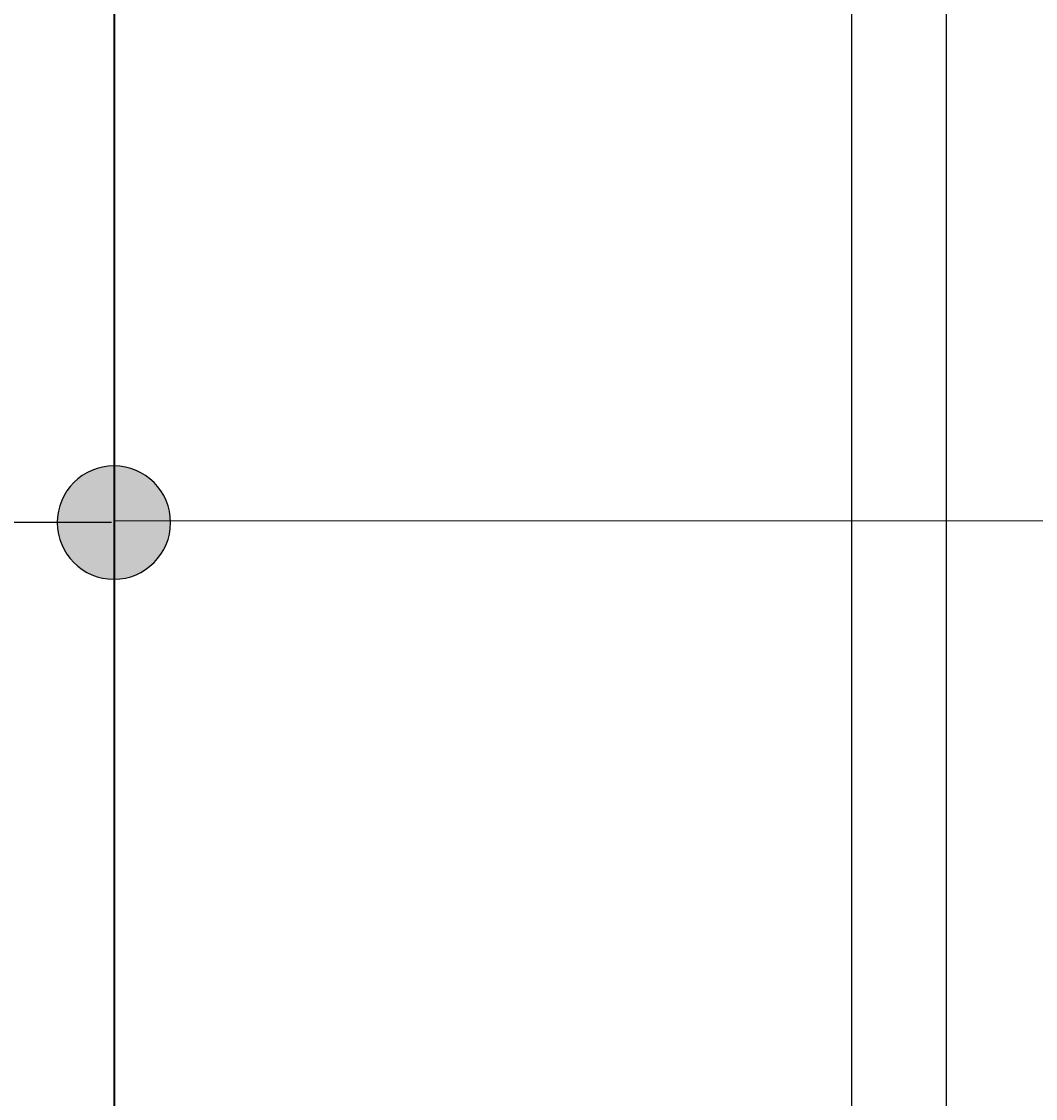
# Model space of a CAD drawing. Units: inches. Extents: x 738 to 1068, y 378 to 757.
# Tile 25 of 41: x 779 to 806, y 578 to 606. Entities that reach past the tile are written whole.
import ezdxf

# ---------------------------------------------------------------- set-up
doc = ezdxf.new("R2010")
doc.units = ezdxf.units.IN
doc.header["$MEASUREMENT"] = 0
for name, color, linetype, lineweight in [('A-ANNO-DIMS', 2, 'Continuous', 18), ('E-CONN', 7, 'Continuous', 25), ('E-CONN-PATT', 7, 'Continuous', 13), ('E-CTRL-WIRE', 7, 'Continuous', 18), ('E-POWR-FEED', 7, 'Continuous', 35)]:
    doc.layers.add(name, color=color, linetype=linetype, lineweight=lineweight)
doc.styles.get("Standard").update_dxf_attribs({"font": 'arial.ttf'})
doc.dimstyles.get("Standard").update_dxf_attribs({"dimtxt": 0.18, "dimasz": 0.18, "dimexe": 0.18, "dimexo": 0.0625, "dimgap": 0.09, "dimtad": 0, "dimtih": 1, "dimtoh": 1, "dimdec": 4, "dimzin": 0, "dimdsep": 46, "dimtxsty": 'Standard', "dimcen": 0.09, "dimadec": 0, "dimazin": 0, "dimtfac": 1, "dimtdec": 4, "dimtofl": 0, "dimtmove": 0, "dimatfit": 3, "dimfxl": 1, "dimtolj": 1, "dimtzin": 0, "dimarcsym": 0})

# ---------------------------------------------------------------- blocks, each defined once
blk = doc.blocks.new('*D22')
at = {"layer": 'A-ANNO-DIMS', "color": 0, "lineweight": -2, "transparency": 16777216}
for p, q in [((781.422, 593.08), (738.194, 593.08)), ((738.374, 592.9), (738.374, 562.422)), ((738.374, 531.581), (738.374, 562.058)), ((781.427, 531.401), (738.194, 531.401))]:
    blk.add_line(p, q, dxfattribs=at)
at = {"layer": 'A-ANNO-DIMS', "color": 0, "transparency": 16777216}
for points in [[(738.344, 592.9), (738.404, 592.9), (738.374, 593.08)], [(738.344, 531.581), (738.404, 531.581), (738.374, 531.401)]]:
    blk.add_solid(points, dxfattribs=at)
at = {"layer": 'Defpoints', "color": 0, "transparency": 16777216}
for p in [(738.374, 593.08), (781.485, 593.08), (781.49, 531.401)]:
    blk.add_point(p, dxfattribs=at)
at = {"layer": 'A-ANNO-DIMS', "color": 0, "transparency": 16777216, "insert": (738.374, 562.24), "char_height": 0.18, "attachment_point": 5}
blk.add_mtext('\\A1;61.68', dxfattribs=at)
blk = doc.blocks.new('*D23')
at = {"layer": 'A-ANNO-DIMS', "color": 0, "lineweight": -2, "transparency": 16777216}
for p, q in [((781.427, 646.985), (738.194, 646.985)), ((738.374, 646.805), (738.374, 620.214)), ((738.374, 593.26), (738.374, 619.85)), ((781.422, 593.08), (738.194, 593.08))]:
    blk.add_line(p, q, dxfattribs=at)
at = {"layer": 'A-ANNO-DIMS', "color": 0, "transparency": 16777216}
for points in [[(738.344, 646.805), (738.404, 646.805), (738.374, 646.985)], [(738.344, 593.26), (738.404, 593.26), (738.374, 593.08)]]:
    blk.add_solid(points, dxfattribs=at)
at = {"layer": 'Defpoints', "color": 0, "transparency": 16777216}
for p in [(738.374, 646.985), (781.49, 646.985), (781.485, 593.08)]:
    blk.add_point(p, dxfattribs=at)
at = {"layer": 'A-ANNO-DIMS', "color": 0, "transparency": 16777216, "insert": (738.374, 620.032), "char_height": 0.18, "attachment_point": 5}
blk.add_mtext('\\A1;53.91', dxfattribs=at)
blk = doc.blocks.new('*D25')
at = {"layer": 'A-ANNO-DIMS', "color": 0, "lineweight": -2, "transparency": 16777216}
for p, q in [((781.49, 646.923), (781.49, 378.239)), ((803.522, 646.923), (803.522, 378.239)), ((781.67, 378.419), (792.111, 378.419)), ((803.342, 378.419), (792.901, 378.419))]:
    blk.add_line(p, q, dxfattribs=at)
at = {"layer": 'A-ANNO-DIMS', "color": 0, "transparency": 16777216}
for points in [[(781.67, 378.449), (781.67, 378.389), (781.49, 378.419)], [(803.342, 378.449), (803.342, 378.389), (803.522, 378.419)]]:
    blk.add_solid(points, dxfattribs=at)
at = {"layer": 'Defpoints', "color": 0, "transparency": 16777216}
for p in [(781.49, 646.985), (803.522, 646.985), (803.522, 378.419)]:
    blk.add_point(p, dxfattribs=at)
at = {"layer": 'A-ANNO-DIMS', "color": 0, "transparency": 16777216, "insert": (792.506, 378.419), "char_height": 0.18, "attachment_point": 5}
blk.add_mtext('\\A1;22.03', dxfattribs=at)
blk = doc.blocks.new('*D31')
at = {"layer": 'A-ANNO-DIMS', "color": 0, "lineweight": -2, "transparency": 16777216}
for p, q in [((781.49, 531.463), (781.49, 756.505)), ((801.022, 531.463), (801.022, 756.505)), ((781.67, 756.325), (790.802, 756.325)), ((800.842, 756.325), (791.71, 756.325))]:
    blk.add_line(p, q, dxfattribs=at)
at = {"layer": 'A-ANNO-DIMS', "color": 0, "transparency": 16777216}
for points in [[(781.67, 756.355), (781.67, 756.295), (781.49, 756.325)], [(800.842, 756.355), (800.842, 756.295), (801.022, 756.325)]]:
    blk.add_solid(points, dxfattribs=at)
at = {"layer": 'Defpoints', "color": 0, "transparency": 16777216}
for p in [(801.022, 756.325), (781.49, 531.401), (801.022, 531.401)]:
    blk.add_point(p, dxfattribs=at)
at = {"layer": 'A-ANNO-DIMS', "color": 0, "transparency": 16777216, "insert": (791.256, 756.325), "char_height": 0.18, "attachment_point": 5}
blk.add_mtext('\\A1;19.532', dxfattribs=at)
blk = doc.blocks.new('*D34')
at = {"layer": 'A-ANNO-DIMS', "color": 0, "lineweight": -2, "transparency": 16777216}
for p, q in [((781.49, 686.266), (781.49, 378.239)), ((830.489, 686.266), (830.489, 378.239)), ((781.67, 378.419), (805.767, 378.419)), ((830.309, 378.419), (806.212, 378.419))]:
    blk.add_line(p, q, dxfattribs=at)
at = {"layer": 'A-ANNO-DIMS', "color": 0, "transparency": 16777216}
for points in [[(781.67, 378.449), (781.67, 378.389), (781.49, 378.419)], [(830.309, 378.449), (830.309, 378.389), (830.489, 378.419)]]:
    blk.add_solid(points, dxfattribs=at)
at = {"layer": 'Defpoints', "color": 0, "transparency": 16777216}
for p in [(781.49, 686.329), (830.489, 686.329), (830.489, 378.419)]:
    blk.add_point(p, dxfattribs=at)
at = {"layer": 'A-ANNO-DIMS', "color": 0, "transparency": 16777216, "insert": (805.99, 378.419), "char_height": 0.18, "attachment_point": 5}
blk.add_mtext('\\A1;49', dxfattribs=at)
blk = doc.blocks.new('*D38')
at = {"layer": 'A-ANNO-DIMS', "color": 0, "lineweight": -2, "transparency": 16777216}
for p, q in [((781.485, 593.017), (781.485, 378.239)), ((887.04, 593.067), (887.04, 378.239)), ((781.665, 378.419), (833.807, 378.419)), ((886.86, 378.419), (834.718, 378.419))]:
    blk.add_line(p, q, dxfattribs=at)
at = {"layer": 'A-ANNO-DIMS', "color": 0, "transparency": 16777216}
for points in [[(781.665, 378.449), (781.665, 378.389), (781.485, 378.419)], [(886.86, 378.449), (886.86, 378.389), (887.04, 378.419)]]:
    blk.add_solid(points, dxfattribs=at)
at = {"layer": 'Defpoints', "color": 0, "transparency": 16777216}
for p in [(781.485, 593.08), (887.04, 593.13), (887.04, 378.419)]:
    blk.add_point(p, dxfattribs=at)
at = {"layer": 'A-ANNO-DIMS', "color": 0, "transparency": 16777216, "insert": (834.263, 378.419), "char_height": 0.18, "attachment_point": 5}
blk.add_mtext('\\A1;105.56', dxfattribs=at)

msp = doc.modelspace()

# ---------------------------------------------------------------- hatches: boundary and pattern name
at = {"layer": 'E-CONN-PATT'}
h = msp.add_hatch(color=256, dxfattribs=at)
h.dxf.hatch_style = 1
h.paths.add_polyline_path([(781.4897, 594.5796, 0.4152031), (779.9846, 593.0796, 0.4152031), (781.4897, 591.5796)])
h.paths.add_polyline_path([(781.4897, 594.5796), (781.4897, 593.1296), (782.9838, 593.1296, 0.4035009)])
h.paths.add_polyline_path([(782.9846, 593.0796, 0.0083343), (782.9838, 593.1296), (781.4897, 593.1296), (781.4897, 591.5796, 0.4132247)])
h.paths.add_polyline_path([(1023.824, 594.6799), (1023.824, 591.7126, 0.3715679), (1025.1031, 593.1962, 0.3715679)])
h.paths.add_polyline_path([(1023.824, 593.1296), (1022.1046, 593.1296, 0.4448148), (1023.824, 591.7126)])
h.paths.add_polyline_path([(1023.824, 594.6799, 0.4581852), (1022.1031, 593.1962, 0.0111068), (1022.1046, 593.1296), (1023.824, 593.1296)])

# ---------------------------------------------------------------- linework, layer by layer
at = {"layer": 'E-CONN'}
msp.add_lwpolyline([(779.9846, 593.0796, 1), (782.9846, 593.0796, 1)], format="xyb", close=True, dxfattribs=at)
at = {"layer": 'E-CTRL-WIRE'}
msp.add_line((781.4897, 593.1296), (887.0404, 593.1296), dxfattribs=at)
at = {"layer": 'E-POWR-FEED'}
msp.add_line((781.4897, 686.329), (781.4897, 437.7164), dxfattribs=at)

# ---------------------------------------------------------------- dimensions: what is measured, and where the dimension line sits
at = {"layer": 'A-ANNO-DIMS'}
for base, p1, p2, override, picture, middle in [((801.0218, 756.3251), (781.4897, 531.4009), (801.0218, 531.4009), {"dimdec": 3, "dimlfac": 1, "dimrnd": 0, "dimzin": 0, "dimdsep": 46, "dimlunit": 2}, '*D31', (791.2557, 756.3251)), ((830.4893, 378.4191), (781.4897, 686.329), (830.4893, 686.329), {"dimdec": 0, "dimlfac": 1, "dimrnd": 0, "dimzin": 0, "dimdsep": 46, "dimlunit": 2}, '*D34', (805.9895, 378.4191)), ((803.5218, 378.4191), (781.4897, 646.9853), (803.5218, 646.9853), {"dimdec": 2, "dimlfac": 1, "dimrnd": 0, "dimzin": 0, "dimdsep": 46, "dimlunit": 2}, '*D25', (792.5057, 378.4191)), ((887.0404, 378.4191), (781.4846, 593.0796), (887.0404, 593.1296), {"dimdec": 2, "dimlfac": 1, "dimrnd": 0, "dimzin": 0, "dimdsep": 46, "dimlunit": 2}, '*D38', (834.2625, 378.4191))]:
    dim = msp.add_linear_dim(base=base, p1=p1, p2=p2, dimstyle='Standard', override=override, dxfattribs=at)
    dim.commit()
    dim.dimension.update_dxf_attribs({"geometry": picture, "text_midpoint": middle})
for base, p1, p2, picture, middle in [((738.3736, 646.9853), (781.4846, 593.0796), (781.4897, 646.9853), '*D23', (738.3736, 620.0325)), ((738.3736, 593.0796), (781.4897, 531.4009), (781.4846, 593.0796), '*D22', (738.3736, 562.2403))]:
    dim = msp.add_linear_dim(base=base, p1=p1, p2=p2, angle=90, dimstyle='Standard', override={"dimdec": 2, "dimlfac": 1, "dimrnd": 0, "dimzin": 0, "dimdsep": 46, "dimlunit": 2}, dxfattribs=at)
    dim.commit()
    dim.dimension.update_dxf_attribs({"geometry": picture, "text_midpoint": middle})

doc.saveas('drawing.dxf')
